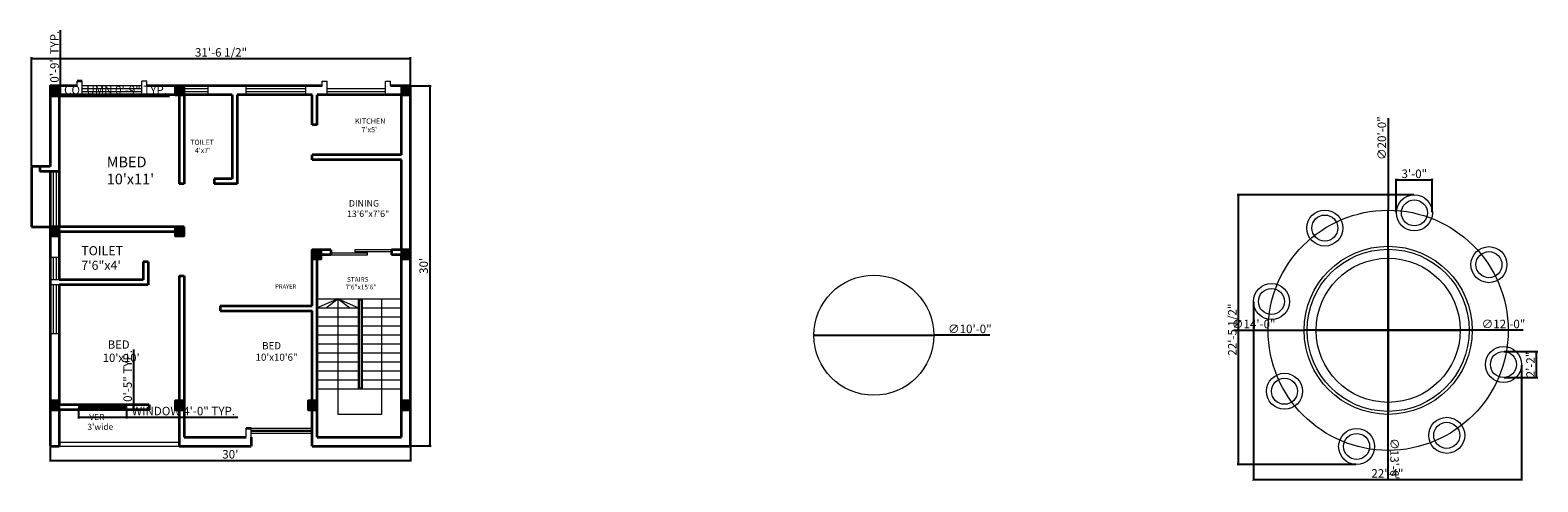
# Model space of a CAD drawing. Units: inches. Extents: x 3799 to 20199, y 1682 to 8087.
# Tile 1 of 30: x 3799 to 5306, y 1682 to 2133. Entities that reach past the tile are written whole.
import ezdxf

# ---------------------------------------------------------------- set-up
doc = ezdxf.new("R2010")
doc.units = ezdxf.units.IN
for name, color, linetype, lineweight in [('A-ANNO-DIMS', 2, 'Continuous', 18), ('A-AREA-IDEN', 7, 'Continuous', 18), ('A-COLS', 251, 'Continuous', 35), ('A-DETL', 7, 'Continuous', 18), ('A-DOOR', 3, 'Continuous', 18), ('A-FLOR-RAIL', 217, 'Continuous', 18), ('A-FLOR-STRS', 41, 'Continuous', 18), ('A-GLAZ', 152, 'Continuous', 18), ('A-WALL', 7, 'Continuous', 35)]:
    doc.layers.add(name, color=color, linetype=linetype, lineweight=lineweight)
doc.styles.get("Standard").update_dxf_attribs({"font": 'arial.ttf'})
doc.dimstyles.new('ISO-25', dxfattribs={"dimtxt": 8.5, "dimasz": 2.5, "dimexe": 1.25, "dimexo": 0.625, "dimtad": 1, "dimdec": 0, "dimlunit": 3, "dimtxsty": 'Standard', "dimblk": 'ARCHTICK', "dimcen": 2.5, "dimadec": 0, "dimazin": 0, "dimtfac": 1, "dimtdec": 0, "dimtmove": 0, "dimatfit": 3, "dimfxl": 1, "dimarcsym": 0})

# ---------------------------------------------------------------- blocks, each defined once
blk = doc.blocks.new('_ArchTick')
at = {"color": 0, "linetype": 'ByBlock', "const_width": 0.15}
blk.add_lwpolyline([(-0.5, -0.5), (0.5, 0.5)], dxfattribs=at)
blk = doc.blocks.new('*D2')
at = {"layer": 'A-ANNO-DIMS', "color": 0, "lineweight": -2, "transparency": 16777216}
for p, q in [((3818.8, 1716.8), (3818.8, 1701.9)), ((3818.8, 1703.1), (4178.8, 1703.1)), ((4178.8, 1716.8), (4178.8, 1701.9))]:
    blk.add_line(p, q, dxfattribs=at)
at = {"layer": 'Defpoints', "color": 0, "transparency": 16777216}
for p in [(3818.8, 1717.5), (4178.8, 1717.5), (4178.8, 1703.1)]:
    blk.add_point(p, dxfattribs=at)
at = {"layer": 'A-ANNO-DIMS', "color": 0, "lineweight": -2, "transparency": 16777216, "xscale": 2.5, "yscale": 2.5, "zscale": 2.5, "rotation": 180}
blk.add_blockref('_ArchTick', (3818.8, 1703.1), dxfattribs=at)
at = {"layer": 'A-ANNO-DIMS', "color": 0, "lineweight": -2, "transparency": 16777216, "xscale": 2.5, "yscale": 2.5, "zscale": 2.5}
blk.add_blockref('_ArchTick', (4178.8, 1703.1), dxfattribs=at)
at = {"layer": 'A-ANNO-DIMS', "color": 0, "transparency": 16777216, "insert": (3998.8, 1708.1), "char_height": 8.5, "attachment_point": 5}
blk.add_mtext("30'", dxfattribs=at)
blk = doc.blocks.new('*D3')
at = {"layer": 'A-ANNO-DIMS', "color": 0, "lineweight": -2, "transparency": 16777216}
for p, q in [((4179.4, 2077.5), (4199.4, 2077.5)), ((4198.2, 2077.5), (4198.2, 1717.5)), ((4179.4, 1717.5), (4199.4, 1717.5))]:
    blk.add_line(p, q, dxfattribs=at)
at = {"layer": 'Defpoints', "color": 0, "transparency": 16777216}
for p in [(4178.8, 2077.5), (4178.8, 1717.5), (4198.2, 1717.5)]:
    blk.add_point(p, dxfattribs=at)
at = {"layer": 'A-ANNO-DIMS', "color": 0, "lineweight": -2, "transparency": 16777216, "xscale": 2.5, "yscale": 2.5, "zscale": 2.5}
for p, rotation in [((4198.2, 2077.5), 90), ((4198.2, 1717.5), 270)]:
    blk.add_blockref('_ArchTick', p, dxfattribs=dict(at, rotation=rotation))
at = {"layer": 'A-ANNO-DIMS', "color": 0, "transparency": 16777216, "insert": (4193.2, 1897.5), "char_height": 8.5, "attachment_point": 5, "rotation": 90}
blk.add_mtext("30'", dxfattribs=at)
blk = doc.blocks.new('*U4')
for radius in [18, 13]:
    blk.add_circle((65.6, 19.3), radius)
blk = doc.blocks.new('*U5')
at = {"layer": 'A-DETL', "color": 0, "linetype": 'ByBlock', "lineweight": -2, "transparency": 16777216}
for p, rotation in [((5241.8, 1917), 134.3437921616318), ((5158.7, 1953.1), 178.6875843232637), ((5276, 1833.1), 90), ((5074.1, 1920.8), 223.0313764848954), ((5233.7, 1741.7), 40.40654513142267), ((5036.1, 1838.6), 267.3751686465272), ((5066.4, 1753.2), 311.718960808159), ((5147.7, 1713.4), 356.062752969791)]:
    blk.add_blockref('*U4', p, dxfattribs=dict(at, rotation=rotation))
blk = doc.blocks.new('WIN-48IN-5IN-FRAME')
for p, q in [((0, 5), (0, 0)), ((48, 3), (0, 3)), ((48, 2), (0, 2)), ((48, 5), (48, 0))]:
    blk.add_line(p, q)
blk = doc.blocks.new('COL-9X9IN')
h = blk.add_hatch(color=256)
h.dxf.hatch_style = 1
h.paths.add_polyline_path([(9, 9), (0, 9), (0, 0), (9, 0)])
blk.add_lwpolyline([(9, 9), (0, 9), (0, 0), (9, 0)], close=True)
blk = doc.blocks.new('*D270')
at = {"layer": 'A-ANNO-DIMS', "color": 0, "lineweight": -2, "transparency": 16777216}
for p, q in [((3818.8, 2067.8), (3818.8, 2065.9)), ((3818.8, 2067.1), (3827.8, 2067.1)), ((3827.8, 2067.8), (3827.8, 2065.9)), ((3827.8, 2067.1), (3938, 2067.1))]:
    blk.add_line(p, q, dxfattribs=at)
at = {"layer": 'Defpoints', "color": 0, "transparency": 16777216}
for p in [(3818.8, 2068.5), (3827.8, 2068.5), (3827.8, 2067.1)]:
    blk.add_point(p, dxfattribs=at)
at = {"layer": 'A-ANNO-DIMS', "color": 0, "lineweight": -2, "transparency": 16777216, "xscale": 2.5, "yscale": 2.5, "zscale": 2.5, "rotation": 180}
blk.add_blockref('_ArchTick', (3818.8, 2067.1), dxfattribs=at)
at = {"layer": 'A-ANNO-DIMS', "color": 0, "lineweight": -2, "transparency": 16777216, "xscale": 2.5, "yscale": 2.5, "zscale": 2.5}
blk.add_blockref('_ArchTick', (3827.8, 2067.1), dxfattribs=at)
at = {"layer": 'A-ANNO-DIMS', "color": 0, "transparency": 16777216, "insert": (3884.1, 2072.1), "char_height": 8.5, "attachment_point": 5}
blk.add_mtext('COLUMN 0\'-9" TYP.', dxfattribs=at)
blk = doc.blocks.new('*D271')
at = {"layer": 'A-ANNO-DIMS', "color": 0, "lineweight": -2, "transparency": 16777216}
for p, q in [((3829.1, 2077.5), (3829.1, 2133)), ((3828.4, 2077.5), (3830.4, 2077.5)), ((3828.4, 2068.5), (3830.4, 2068.5)), ((3829.1, 2068.5), (3829.1, 2077.5))]:
    blk.add_line(p, q, dxfattribs=at)
at = {"layer": 'Defpoints', "color": 0, "transparency": 16777216}
for p in [(3827.8, 2077.5), (3827.8, 2068.5), (3829.1, 2077.5)]:
    blk.add_point(p, dxfattribs=at)
at = {"layer": 'A-ANNO-DIMS', "color": 0, "lineweight": -2, "transparency": 16777216, "xscale": 2.5, "yscale": 2.5, "zscale": 2.5}
for p, rotation in [((3829.1, 2077.5), 90), ((3829.1, 2068.5), 270)]:
    blk.add_blockref('_ArchTick', p, dxfattribs=dict(at, rotation=rotation))
at = {"layer": 'A-ANNO-DIMS', "color": 0, "transparency": 16777216, "insert": (3824.2, 2106.5), "char_height": 8.5, "attachment_point": 5, "rotation": 90}
blk.add_mtext('0\'-9" TYP.', dxfattribs=at)
blk = doc.blocks.new('*D324')
at = {"layer": 'A-ANNO-DIMS', "color": 0, "lineweight": -2, "transparency": 16777216}
for p, q in [((3847.1, 1752.8), (3847.1, 1745)), ((3895.1, 1752.8), (3895.1, 1745)), ((3847.1, 1746.3), (3895.1, 1746.3)), ((3895.1, 1746.3), (4006.4, 1746.3))]:
    blk.add_line(p, q, dxfattribs=at)
at = {"layer": 'Defpoints', "color": 0, "transparency": 16777216}
for p in [(3847.1, 1753.5), (3895.1, 1753.5), (3895.1, 1746.3)]:
    blk.add_point(p, dxfattribs=at)
at = {"layer": 'A-ANNO-DIMS', "color": 0, "lineweight": -2, "transparency": 16777216, "xscale": 2.5, "yscale": 2.5, "zscale": 2.5, "rotation": 180}
blk.add_blockref('_ArchTick', (3847.1, 1746.3), dxfattribs=at)
at = {"layer": 'A-ANNO-DIMS', "color": 0, "lineweight": -2, "transparency": 16777216, "xscale": 2.5, "yscale": 2.5, "zscale": 2.5}
blk.add_blockref('_ArchTick', (3895.1, 1746.3), dxfattribs=at)
at = {"layer": 'A-ANNO-DIMS', "color": 0, "transparency": 16777216, "insert": (3952, 1751.3), "char_height": 8.5, "attachment_point": 5}
blk.add_mtext('WINDOW 4\'-0" TYP.', dxfattribs=at)
blk = doc.blocks.new('*D325')
at = {"layer": 'A-ANNO-DIMS', "color": 0, "lineweight": -2, "transparency": 16777216}
for p, q in [((3902.3, 1758.5), (3902.3, 1814)), ((3895.7, 1758.5), (3903.6, 1758.5)), ((3895.7, 1753.5), (3903.6, 1753.5)), ((3902.3, 1753.5), (3902.3, 1758.5))]:
    blk.add_line(p, q, dxfattribs=at)
at = {"layer": 'Defpoints', "color": 0, "transparency": 16777216}
for p in [(3895.1, 1758.5), (3895.1, 1753.5), (3902.3, 1758.5)]:
    blk.add_point(p, dxfattribs=at)
at = {"layer": 'A-ANNO-DIMS', "color": 0, "lineweight": -2, "transparency": 16777216, "xscale": 2.5, "yscale": 2.5, "zscale": 2.5}
for p, rotation in [((3902.3, 1758.5), 90), ((3902.3, 1753.5), 270)]:
    blk.add_blockref('_ArchTick', p, dxfattribs=dict(at, rotation=rotation))
at = {"layer": 'A-ANNO-DIMS', "color": 0, "transparency": 16777216, "insert": (3897.3, 1787.5), "char_height": 8.5, "attachment_point": 5, "rotation": 90}
blk.add_mtext('0\'-5" TYP.', dxfattribs=at)
blk = doc.blocks.new('*D360')
at = {"layer": 'A-ANNO-DIMS', "color": 0, "lineweight": -2, "transparency": 16777216}
for p, q in [((5164.1, 1951), (5164.1, 1984.6)), ((5164.1, 1983.4), (5200.1, 1983.4)), ((5200.1, 1951), (5200.1, 1984.6))]:
    blk.add_line(p, q, dxfattribs=at)
at = {"layer": 'Defpoints', "color": 0, "transparency": 16777216}
for p in [(5200.1, 1983.4), (5164.1, 1950.4), (5200.1, 1950.4)]:
    blk.add_point(p, dxfattribs=at)
at = {"layer": 'A-ANNO-DIMS', "color": 0, "lineweight": -2, "transparency": 16777216, "xscale": 2.5, "yscale": 2.5, "zscale": 2.5, "rotation": 180}
blk.add_blockref('_ArchTick', (5164.1, 1983.4), dxfattribs=at)
at = {"layer": 'A-ANNO-DIMS', "color": 0, "lineweight": -2, "transparency": 16777216, "xscale": 2.5, "yscale": 2.5, "zscale": 2.5}
blk.add_blockref('_ArchTick', (5200.1, 1983.4), dxfattribs=at)
at = {"layer": 'A-ANNO-DIMS', "color": 0, "transparency": 16777216, "insert": (5182.1, 1988.4), "char_height": 8.5, "attachment_point": 5}
blk.add_mtext('3\'-0"', dxfattribs=at)
blk = doc.blocks.new('*D361')
at = {"layer": 'A-ANNO-DIMS', "color": 0, "lineweight": -2, "transparency": 16777216}
for p, q in [((5271.8, 1811.9), (5305.4, 1811.9)), ((5304.2, 1785.9), (5304.2, 1811.9)), ((5271.8, 1785.9), (5305.4, 1785.9))]:
    blk.add_line(p, q, dxfattribs=at)
at = {"layer": 'Defpoints', "color": 0, "transparency": 16777216}
for p in [(5271.2, 1811.9), (5304.2, 1811.9), (5271.2, 1785.9)]:
    blk.add_point(p, dxfattribs=at)
at = {"layer": 'A-ANNO-DIMS', "color": 0, "lineweight": -2, "transparency": 16777216, "xscale": 2.5, "yscale": 2.5, "zscale": 2.5}
for p, rotation in [((5304.2, 1811.9), 90), ((5304.2, 1785.9), 270)]:
    blk.add_blockref('_ArchTick', p, dxfattribs=dict(at, rotation=rotation))
at = {"layer": 'A-ANNO-DIMS', "color": 0, "transparency": 16777216, "insert": (5299.3, 1798.9), "char_height": 8.5, "attachment_point": 5, "rotation": 90}
blk.add_mtext('2\'-2"', dxfattribs=at)
blk = doc.blocks.new('*D362')
at = {"layer": 'A-ANNO-DIMS', "color": 0, "lineweight": -2, "transparency": 16777216}
for p, q in [((5021.3, 1861.4), (5021.3, 1682.9)), ((5289.2, 1798.3), (5289.2, 1682.9)), ((5021.3, 1684.1), (5289.2, 1684.1))]:
    blk.add_line(p, q, dxfattribs=at)
at = {"layer": 'Defpoints', "color": 0, "transparency": 16777216}
for p in [(5021.3, 1862), (5289.2, 1798.9), (5289.2, 1684.1)]:
    blk.add_point(p, dxfattribs=at)
at = {"layer": 'A-ANNO-DIMS', "color": 0, "lineweight": -2, "transparency": 16777216, "xscale": 2.5, "yscale": 2.5, "zscale": 2.5, "rotation": 180}
blk.add_blockref('_ArchTick', (5021.3, 1684.1), dxfattribs=at)
at = {"layer": 'A-ANNO-DIMS', "color": 0, "lineweight": -2, "transparency": 16777216, "xscale": 2.5, "yscale": 2.5, "zscale": 2.5}
blk.add_blockref('_ArchTick', (5289.2, 1684.1), dxfattribs=at)
at = {"layer": 'A-ANNO-DIMS', "color": 0, "transparency": 16777216, "insert": (5155.2, 1689), "char_height": 8.5, "attachment_point": 5}
blk.add_mtext('22\'-4"', dxfattribs=at)
blk = doc.blocks.new('*D363')
at = {"layer": 'A-ANNO-DIMS', "color": 0, "lineweight": -2, "transparency": 16777216}
for p, q in [((5181.5, 1968.4), (5005, 1968.4)), ((5006.3, 1699.1), (5006.3, 1968.4)), ((5123.8, 1699.1), (5005, 1699.1))]:
    blk.add_line(p, q, dxfattribs=at)
at = {"layer": 'Defpoints', "color": 0, "transparency": 16777216}
for p in [(5006.3, 1968.4), (5182.1, 1968.4), (5124.4, 1699.1)]:
    blk.add_point(p, dxfattribs=at)
at = {"layer": 'A-ANNO-DIMS', "color": 0, "lineweight": -2, "transparency": 16777216, "xscale": 2.5, "yscale": 2.5, "zscale": 2.5}
for p, rotation in [((5006.3, 1968.4), 90), ((5006.3, 1699.1), 270)]:
    blk.add_blockref('_ArchTick', p, dxfattribs=dict(at, rotation=rotation))
at = {"layer": 'A-ANNO-DIMS', "color": 0, "transparency": 16777216, "insert": (5001.3, 1833.8), "char_height": 8.5, "attachment_point": 5, "rotation": 90}
blk.add_mtext('22\'-5 1/2"', dxfattribs=at)
blk = doc.blocks.new('*D366')
at = {"layer": 'A-ANNO-DIMS', "color": 0, "lineweight": -2, "transparency": 16777216}
for p, q in [((3800.2, 1997.5), (3800.2, 2105.9)), ((3800.2, 2104.7), (4178.8, 2104.7)), ((4178.8, 2078.1), (4178.8, 2105.9))]:
    blk.add_line(p, q, dxfattribs=at)
at = {"layer": 'Defpoints', "color": 0, "transparency": 16777216}
for p in [(4178.8, 2104.7), (4178.8, 2077.5), (3800.2, 1996.9)]:
    blk.add_point(p, dxfattribs=at)
at = {"layer": 'A-ANNO-DIMS', "color": 0, "lineweight": -2, "transparency": 16777216, "xscale": 2.5, "yscale": 2.5, "zscale": 2.5, "rotation": 180}
blk.add_blockref('_ArchTick', (3800.2, 2104.7), dxfattribs=at)
at = {"layer": 'A-ANNO-DIMS', "color": 0, "lineweight": -2, "transparency": 16777216, "xscale": 2.5, "yscale": 2.5, "zscale": 2.5}
blk.add_blockref('_ArchTick', (4178.8, 2104.7), dxfattribs=at)
at = {"layer": 'A-ANNO-DIMS', "color": 0, "transparency": 16777216, "insert": (3989.5, 2109.7), "char_height": 8.5, "attachment_point": 5}
blk.add_mtext('31\'-6 1/2"', dxfattribs=at)
blk = doc.blocks.new('*D379')
at = {"layer": 'A-ANNO-DIMS', "color": 0, "lineweight": -2, "transparency": 16777216}
for p in [(4581.9, 1828.2), (4757.8, 1828.2)]:
    blk.add_line(p, (4701.9, 1828.2), dxfattribs=at)
at = {"layer": 'Defpoints', "color": 0, "transparency": 16777216}
for p in [(4581.9, 1828.2), (4701.9, 1828.2)]:
    blk.add_point(p, dxfattribs=at)
at = {"layer": 'A-ANNO-DIMS', "color": 0, "lineweight": -2, "transparency": 16777216, "xscale": 2.5, "yscale": 2.5, "zscale": 2.5}
for p, rotation in [((4581.9, 1828.2), 359.9997507633592), ((4701.9, 1828.2), 179.9997507633592)]:
    blk.add_blockref('_ArchTick', p, dxfattribs=dict(at, rotation=rotation))
at = {"layer": 'A-ANNO-DIMS', "color": 0, "transparency": 16777216, "insert": (4737.9, 1833.4), "char_height": 8.5, "attachment_point": 5, "rotation": 359.9998}
blk.add_mtext('∅10\'-0"', dxfattribs=at)
blk = doc.blocks.new('*D380')
at = {"layer": 'A-ANNO-DIMS', "color": 0, "lineweight": -2, "transparency": 16777216}
for p in [(5156, 2045), (5156, 1713.1)]:
    blk.add_line(p, (5156, 1953.1), dxfattribs=at)
at = {"layer": 'Defpoints', "color": 0, "transparency": 16777216}
for p in [(5156, 1953.1), (5156, 1713.1)]:
    blk.add_point(p, dxfattribs=at)
at = {"layer": 'A-ANNO-DIMS', "color": 0, "lineweight": -2, "transparency": 16777216, "xscale": 2.5, "yscale": 2.5, "zscale": 2.5}
for p, rotation in [((5156, 1953.1), 270), ((5156, 1713.1), 90)]:
    blk.add_blockref('_ArchTick', p, dxfattribs=dict(at, rotation=rotation))
at = {"layer": 'A-ANNO-DIMS', "color": 0, "transparency": 16777216, "insert": (5150.7, 2025.1), "char_height": 8.5, "attachment_point": 5, "rotation": 90}
blk.add_mtext('∅20\'-0"', dxfattribs=at)
blk = doc.blocks.new('*D381')
at = {"layer": 'A-ANNO-DIMS', "color": 0, "lineweight": -2, "transparency": 16777216}
for p in [(5001.7, 1833.1), (5240, 1833.1)]:
    blk.add_line(p, (5072, 1833.1), dxfattribs=at)
at = {"layer": 'Defpoints', "color": 0, "transparency": 16777216}
for p in [(5072, 1833.1), (5240, 1833.1)]:
    blk.add_point(p, dxfattribs=at)
at = {"layer": 'A-ANNO-DIMS', "color": 0, "lineweight": -2, "transparency": 16777216, "xscale": 2.5, "yscale": 2.5, "zscale": 2.5}
blk.add_blockref('_ArchTick', (5072, 1833.1), dxfattribs=at)
at = {"layer": 'A-ANNO-DIMS', "color": 0, "lineweight": -2, "transparency": 16777216, "xscale": 2.5, "yscale": 2.5, "zscale": 2.5, "rotation": 180}
blk.add_blockref('_ArchTick', (5240, 1833.1), dxfattribs=at)
at = {"layer": 'A-ANNO-DIMS', "color": 0, "transparency": 16777216, "insert": (5021.6, 1838.3), "char_height": 8.5, "attachment_point": 5}
blk.add_mtext('∅14\'-0"', dxfattribs=at)
blk = doc.blocks.new('*D382')
at = {"layer": 'A-ANNO-DIMS', "color": 0, "lineweight": -2, "transparency": 16777216}
for p in [(5156, 1914.1), (5156, 1683.7)]:
    blk.add_line(p, (5156, 1752.1), dxfattribs=at)
at = {"layer": 'Defpoints', "color": 0, "transparency": 16777216}
for p in [(5156, 1914.1), (5156, 1752.1)]:
    blk.add_point(p, dxfattribs=at)
at = {"layer": 'A-ANNO-DIMS', "color": 0, "lineweight": -2, "transparency": 16777216, "xscale": 2.5, "yscale": 2.5, "zscale": 2.5}
for p, rotation in [((5156, 1914.1), 270.0000643693325), ((5156, 1752.1), 90.00006436933245)]:
    blk.add_blockref('_ArchTick', p, dxfattribs=dict(at, rotation=rotation))
at = {"layer": 'A-ANNO-DIMS', "color": 0, "transparency": 16777216, "insert": (5161.2, 1703.5), "char_height": 8.5, "attachment_point": 5, "rotation": 270.0001}
blk.add_mtext('∅13\'-6"', dxfattribs=at)
blk = doc.blocks.new('*D383')
at = {"layer": 'A-ANNO-DIMS', "color": 0, "lineweight": -2, "transparency": 16777216}
for p in [(5084, 1833.1), (5291, 1833.1)]:
    blk.add_line(p, (5228, 1833.1), dxfattribs=at)
at = {"layer": 'Defpoints', "color": 0, "transparency": 16777216}
for p in [(5084, 1833.1), (5228, 1833.1)]:
    blk.add_point(p, dxfattribs=at)
at = {"layer": 'A-ANNO-DIMS', "color": 0, "lineweight": -2, "transparency": 16777216, "xscale": 2.5, "yscale": 2.5, "zscale": 2.5}
for p, rotation in [((5084, 1833.1), 359.9999514577424), ((5228, 1833.1), 179.9999514577424)]:
    blk.add_blockref('_ArchTick', p, dxfattribs=dict(at, rotation=rotation))
at = {"layer": 'A-ANNO-DIMS', "color": 0, "transparency": 16777216, "insert": (5271.2, 1838.3), "char_height": 8.5, "attachment_point": 5, "rotation": 360}
blk.add_mtext('∅12\'-0"', dxfattribs=at)

msp = doc.modelspace()

# ---------------------------------------------------------------- linework, layer by layer
at = {"layer": 'A-DETL'}
for centre, radius in [((5155.95, 1833.1), 120), ((5155.95, 1833.1), 84), ((5155.95, 1833.1), 81), ((5155.95, 1833.1), 72), ((4641.93, 1828.16), 60)]:
    msp.add_circle(centre, radius, dxfattribs=at)
at = {"layer": 'A-DOOR'}
for p, q in [((4099.28, 1910.47), (4135.83, 1910.47)), ((4099.28, 1908.47), (4135.83, 1908.47)), ((4159.93, 1913.47), (4123.17, 1913.47)), ((4123.17, 1913.47), (4123.17, 1911.47)), ((4159.93, 1911.47), (4123.17, 1911.47)), ((4135.83, 1908.47), (4135.83, 1910.47))]:
    msp.add_line(p, q, dxfattribs=at)
at = {"layer": 'A-FLOR-RAIL'}
for p, q in [((3827.77, 1721.47), (3947.77, 1721.47)), ((3827.77, 1717.47), (3947.77, 1717.47))]:
    msp.add_line(p, q, dxfattribs=at)
at = {"layer": 'A-FLOR-STRS'}
for p, q in [((4085.77, 1864.58), (4169.77, 1864.58)), ((4106.74, 1864.58), (4085.77, 1855.58)), ((4085.77, 1855.58), (4126.77, 1855.58)), ((4106.74, 1864.58), (4094.8, 1855.58)), ((4106.74, 1748.85), (4106.74, 1864.58)), ((4106.74, 1864.58), (4126.77, 1855.58)), ((4106.74, 1864.58), (4118.34, 1855.58)), ((4126.77, 1774.58), (4126.77, 1864.58)), ((4127.77, 1775.58), (4127.77, 1863.58)), ((4127.77, 1863.58), (4129.77, 1863.58)), ((4129.77, 1775.58), (4129.77, 1863.58)), ((4130.77, 1774.58), (4130.77, 1864.58)), ((4130.77, 1855.58), (4169.77, 1855.58)), ((4150.03, 1864.58), (4150.03, 1748.85)), ((4085.77, 1846.58), (4126.77, 1846.58)), ((4130.77, 1846.58), (4169.77, 1846.58)), ((4085.77, 1837.58), (4126.77, 1837.58)), ((4085.77, 1828.58), (4126.77, 1828.58)), ((4130.77, 1837.58), (4169.77, 1837.58)), ((4130.77, 1828.58), (4169.77, 1828.58)), ((4085.77, 1819.58), (4126.77, 1819.58)), ((4085.77, 1810.58), (4126.77, 1810.58)), ((4130.77, 1819.58), (4169.77, 1819.58)), ((4130.77, 1810.58), (4169.77, 1810.58)), ((4085.77, 1801.58), (4126.77, 1801.58)), ((4130.77, 1801.58), (4169.77, 1801.58)), ((4085.77, 1792.58), (4126.77, 1792.58)), ((4085.77, 1783.58), (4126.77, 1783.58)), ((4130.77, 1792.58), (4169.77, 1792.58)), ((4130.77, 1783.58), (4169.77, 1783.58)), ((4085.77, 1774.58), (4169.77, 1774.58)), ((4127.77, 1775.58), (4129.77, 1775.58)), ((4150.03, 1748.85), (4106.74, 1748.85))]:
    msp.add_line(p, q, dxfattribs=at)
at = {"layer": 'A-GLAZ'}
for p, q in [((3845.89, 2077.47), (3845.89, 2082.18)), ((3850.89, 2068.47), (3850.89, 2082.18)), ((3910.28, 2068.47), (3910.28, 2082.18)), ((3915.28, 2082.18), (3910.28, 2082.18)), ((3915.28, 2077.47), (3915.28, 2082.18)), ((4090.62, 2077.47), (4090.62, 2082.18)), ((4090.62, 2082.18), (4095.62, 2082.18)), ((4095.62, 2068.47), (4095.62, 2082.18)), ((4154.03, 2068.47), (4154.03, 2082.18)), ((4154.03, 2082.18), (4159.03, 2082.18)), ((4159.03, 2077.47), (4159.03, 2082.18)), ((3910.28, 2077.47), (3850.89, 2077.47)), ((3910.28, 2074.47), (3850.89, 2074.47)), ((3910.28, 2071.47), (3850.89, 2071.47)), ((3976.33, 2074.47), (3952.75, 2074.47)), ((3976.33, 2071.47), (3952.77, 2071.47)), ((3976.33, 2077.47), (3976.33, 2068.47)), ((4014.74, 2068.47), (4014.74, 2077.47)), ((4074.26, 2074.47), (4014.74, 2074.47)), ((4074.26, 2071.47), (4014.74, 2071.47)), ((4074.26, 2068.47), (4074.26, 2077.47)), ((4154.03, 2074.47), (4095.62, 2074.47)), ((4154.03, 2071.47), (4095.62, 2071.47)), ((3821.77, 1991.87), (3821.77, 1936.47)), ((3824.77, 1991.87), (3824.77, 1936.47)), ((3827.77, 1905.89), (3818.77, 1905.89)), ((3821.77, 1905.89), (3821.77, 1883.47)), ((3824.77, 1905.89), (3824.77, 1883.47)), ((3827.77, 1883.47), (3818.77, 1883.47)), ((3827.77, 1878.47), (3818.77, 1878.47)), ((3821.77, 1878.47), (3821.77, 1829.54)), ((3824.77, 1878.47), (3824.77, 1829.54)), ((3827.77, 1829.54), (3818.77, 1829.54)), ((4014.77, 1726.47), (4014.77, 1735.44)), ((4019.77, 1726.47), (4019.77, 1735.44)), ((4019.77, 1735.44), (4080.77, 1735.44)), ((4019.77, 1733.44), (4080.77, 1733.44)), ((4019.77, 1732.44), (4080.77, 1732.44)), ((4019.77, 1730.44), (4080.77, 1730.44))]:
    msp.add_line(p, q, dxfattribs=at)
at = {"layer": 'A-WALL'}
for p, q in [((3850.89, 2082.18), (3845.89, 2082.18)), ((3818.77, 2077.47), (3818.77, 1996.87)), ((3845.89, 2077.47), (3818.77, 2077.47)), ((3821.77, 2077.47), (3821.77, 2068.47)), ((3827.77, 2068.47), (3827.77, 1936.47)), ((3947.77, 2068.47), (3827.77, 2068.47)), ((4090.62, 2077.47), (3915.28, 2077.47)), ((3947.77, 2068.47), (3947.77, 1979.47)), ((3952.77, 2068.47), (3952.77, 1984.47)), ((4000.77, 2068.47), (3952.77, 2068.47)), ((4000.77, 2068.47), (4000.77, 1984.47)), ((4005.77, 2068.47), (4005.77, 1979.47)), ((4080.77, 2068.47), (4005.77, 2068.47)), ((4080.77, 2038.47), (4080.77, 2068.47)), ((4169.77, 2068.47), (4085.77, 2068.47)), ((4085.77, 2038.47), (4085.77, 2068.47)), ((4178.77, 2077.47), (4159.03, 2077.47)), ((4178.77, 2074.47), (4169.77, 2074.47)), ((4169.77, 2008.47), (4169.77, 2068.47)), ((4178.77, 1717.47), (4178.77, 2077.47)), ((4085.77, 2038.47), (4080.77, 2038.47)), ((4080.77, 2003.47), (4080.77, 2008.47)), ((4085.77, 2008.47), (4080.77, 2008.47)), ((4169.77, 2008.47), (4085.77, 2008.47)), ((3808.35, 1996.87), (3800.15, 1996.87)), ((3800.15, 1996.87), (3800.15, 1936.47)), ((3818.77, 1996.87), (3808.35, 1996.87)), ((3808.35, 1996.87), (3808.35, 1991.87)), ((3827.77, 1991.87), (3808.35, 1991.87)), ((3818.77, 1991.87), (3818.77, 1717.47)), ((4169.77, 2003.47), (4080.77, 2003.47)), ((4169.77, 1913.47), (4169.77, 2003.47)), ((3952.77, 1979.47), (3947.77, 1979.47)), ((3952.77, 1984.47), (3952.77, 1979.47)), ((4000.77, 1984.47), (3982.77, 1984.47)), ((3982.77, 1984.47), (3982.77, 1979.47)), ((4005.77, 1979.47), (3982.77, 1979.47)), ((3800.15, 1936.47), (3818.77, 1936.47)), ((3952.77, 1936.47), (3827.77, 1936.47)), ((3952.77, 1931.47), (3827.77, 1931.47)), ((3827.77, 1931.47), (3827.77, 1883.47)), ((3952.77, 1931.47), (3952.77, 1936.47)), ((3911.77, 1901.47), (3911.77, 1883.47)), ((3916.77, 1901.47), (3911.77, 1901.47)), ((3916.77, 1901.47), (3916.77, 1878.47)), ((4080.77, 1857.47), (4080.77, 1913.47)), ((4099.28, 1913.47), (4080.77, 1913.47)), ((4085.77, 1726.47), (4085.77, 1908.47)), ((4099.28, 1908.47), (4085.77, 1908.47)), ((4099.28, 1913.47), (4099.28, 1908.47)), ((4169.77, 1913.47), (4159.93, 1913.47)), ((4159.93, 1913.47), (4159.93, 1908.47)), ((4169.77, 1908.47), (4159.93, 1908.47)), ((4169.77, 1726.47), (4169.77, 1908.47)), ((3947.77, 1887.43), (3947.77, 1758.47)), ((3947.77, 1887.43), (3952.77, 1887.43)), ((3952.77, 1887.43), (3952.77, 1726.47)), ((3911.77, 1883.47), (3827.77, 1883.47)), ((3916.77, 1878.47), (3827.77, 1878.47)), ((3827.77, 1878.47), (3827.77, 1758.47)), ((3988.77, 1857.47), (4080.77, 1857.47)), ((3988.77, 1857.47), (3988.77, 1852.47)), ((3988.77, 1852.47), (4080.77, 1852.47)), ((4080.77, 1717.47), (4080.77, 1852.47)), ((3917.77, 1758.47), (3827.77, 1758.47)), ((3917.77, 1753.47), (3827.77, 1753.47)), ((3827.77, 1753.47), (3827.77, 1722.47)), ((3917.77, 1758.47), (3917.77, 1753.47)), ((3947.77, 1758.47), (3947.77, 1753.47)), ((3947.77, 1753.47), (3947.77, 1717.47)), ((4014.77, 1735.44), (4019.77, 1735.44)), ((3827.77, 1722.47), (3827.77, 1717.47)), ((3952.77, 1726.47), (4014.77, 1726.47)), ((4019.77, 1726.47), (4019.77, 1717.47)), ((4085.77, 1726.47), (4169.77, 1726.47)), ((3818.77, 1717.47), (3827.77, 1717.47)), ((3947.77, 1717.47), (4019.77, 1717.47)), ((4080.77, 1717.47), (4178.77, 1717.47))]:
    msp.add_line(p, q, dxfattribs=at)

# ---------------------------------------------------------------- block references
at = {"layer": 'A-COLS'}
for p in [(3818.77, 2068.47), (3943.75, 2068.47), (4169.77, 2068.47), (3818.77, 1927.47), (3943.78, 1927.47), (4080.77, 1904.37), (4169.77, 1904.47), (3818.77, 1753.47), (3943.77, 1753.47), (4076.77, 1753.47), (4169.77, 1753.47)]:
    msp.add_blockref('COL-9X9IN', p, dxfattribs=at)
at = {"layer": 'A-DETL'}
msp.add_blockref('*U5', (0, 0), dxfattribs=at)
at = {"layer": 'A-GLAZ'}
msp.add_blockref('WIN-48IN-5IN-FRAME', (3847.11, 1753.47), dxfattribs=at)

# ---------------------------------------------------------------- texts
at = {"layer": 'A-AREA-IDEN'}
for s, height, p in [('KITCHEN', 5.296, (4123.41, 2039.49)), ("    7'x5'", 5.296, (4123.41, 2030.98)), ('TOILET', 5.117, (3958.78, 2018.46)), ('MBED', 10.616, (3875.31, 1995.98)), ("   4'x7'", 5.117, (3958.78, 2010.24)), ("10'x11'", 10.616, (3875.32, 1978.92)), (' DINING', 6.485, (4115.36, 1956.71)), ('13\'6"x7\'6"', 6.485, (4115.37, 1946.29)), ('TOILET', 9.087, (3849.85, 1908.11)), ('7\'6"x4\'', 9.087, (3849.85, 1893.52)), (' STAIRS', 4.733, (4113.98, 1881.55)), ('PRAYER', 4.244, (4043.67, 1874.78)), ('7\'6"x15\'6"', 4.733, (4113.98, 1873.94)), ("10'x10'", 8.245, (3871.36, 1801.49)), ('  BED', 8.245, (3871.35, 1814.73)), ('10\'x10\'6"', 7.162, (4024.02, 1802.62)), ('   BED', 7.162, (4024.02, 1814.13)), (' VER', 6.14, (3855.95, 1743.45)), ("3'wide", 6.14, (3855.96, 1733.58))]:
    msp.add_text(s, height=height, rotation=0.03333, dxfattribs=at).set_placement(p)

# ---------------------------------------------------------------- dimensions: what is measured, and where the dimension line sits
at = {"layer": 'A-ANNO-DIMS'}
for base, p1, p2, picture, middle in [((3829.12, 2077.47), (3827.77, 2068.47), (3827.77, 2077.47), '*D271', (3824.16, 2106.51)), ((3902.31, 1758.47), (3895.11, 1753.47), (3895.11, 1758.47), '*D325', (3897.35, 1787.51))]:
    dim = msp.add_linear_dim(base=base, p1=p1, p2=p2, angle=90, text='<> TYP.', dimstyle='ISO-25', override={"dimdec": 1, "dimlfac": 1, "dimrnd": 0, "dimzin": 1, "dimdsep": 46, "dimlunit": 4, "dimfrac": 2}, dxfattribs=at)
    dim.commit()
    dim.dimension.update_dxf_attribs({"geometry": picture, "text_midpoint": middle})
for base, p1, p2, override, picture, middle in [((4178.77, 2104.68), (3800.15, 1996.87), (4178.77, 2077.47), {"dimdec": 1, "dimlfac": 1, "dimrnd": 0, "dimzin": 1, "dimdsep": 46, "dimlunit": 4, "dimfrac": 2}, '*D366', (3989.46, 2109.7)), ((5200.15, 1983.4), (5164.15, 1950.4), (5200.15, 1950.4), {"dimdec": 1, "dimlfac": 1, "dimrnd": 0, "dimzin": 1, "dimdsep": 46, "dimlunit": 4, "dimfrac": 2}, '*D360', (5182.15, 1988.36)), ((5289.17, 1684.13), (5021.29, 1861.98), (5289.17, 1798.92), {"dimdec": 1, "dimlfac": 1, "dimrnd": 0, "dimzin": 1, "dimdsep": 46, "dimlunit": 4, "dimfrac": 2}, '*D362', (5155.23, 1689.02)), ((4178.77, 1703.15), (3818.77, 1717.47), (4178.77, 1717.47), {"dimclrd": 0, "dimclre": 0, "dimclrt": 0}, '*D2', (3998.77, 1708.11))]:
    dim = msp.add_linear_dim(base=base, p1=p1, p2=p2, dimstyle='ISO-25', override=override, dxfattribs=at)
    dim.commit()
    dim.dimension.update_dxf_attribs({"geometry": picture, "text_midpoint": middle})
for base, p1, p2, text, picture, middle in [((3827.77, 2067.12), (3818.77, 2068.47), (3827.77, 2068.47), 'COLUMN <> TYP.', '*D270', (3884.13, 2072.15)), ((3895.11, 1746.27), (3847.11, 1753.47), (3895.11, 1753.47), 'WINDOW <> TYP.', '*D324', (3952.02, 1751.3))]:
    dim = msp.add_linear_dim(base=base, p1=p1, p2=p2, text=text, dimstyle='ISO-25', override={"dimdec": 1, "dimlfac": 1, "dimrnd": 0, "dimzin": 1, "dimdsep": 46, "dimlunit": 4, "dimfrac": 2}, dxfattribs=at)
    dim.commit()
    dim.dimension.update_dxf_attribs({"geometry": picture, "text_midpoint": middle})
for base, p1, p2, override, picture, middle in [((4198.17, 1717.47), (4178.77, 2077.47), (4178.77, 1717.47), {"dimclrd": 0, "dimclre": 0, "dimclrt": 0}, '*D3', (4193.2, 1897.47)), ((5006.29, 1968.4), (5124.41, 1699.13), (5182.15, 1968.4), {"dimdec": 1, "dimlfac": 1, "dimrnd": 0, "dimzin": 1, "dimdsep": 46, "dimlunit": 4, "dimfrac": 2}, '*D363', (5001.27, 1833.76)), ((5304.17, 1811.92), (5271.17, 1785.92), (5271.17, 1811.92), {"dimdec": 1, "dimlfac": 1, "dimrnd": 0, "dimzin": 1, "dimdsep": 46, "dimlunit": 4, "dimfrac": 2}, '*D361', (5299.28, 1798.92))]:
    dim = msp.add_linear_dim(base=base, p1=p1, p2=p2, angle=90, dimstyle='ISO-25', override=override, dxfattribs=at)
    dim.commit()
    dim.dimension.update_dxf_attribs({"geometry": picture, "text_midpoint": middle})
for p1, p2, picture, middle in [((5155.95, 1713.1), (5155.95, 1953.1), '*D380', (5155.95, 2025.1)), ((5155.95, 1914.1), (5155.95, 1752.1), '*D382', (5155.95, 1703.5)), ((4581.93, 1828.16), (4701.93, 1828.16), '*D379', (4737.93, 1828.16)), ((5239.95, 1833.1), (5071.95, 1833.1), '*D381', (5021.55, 1833.1)), ((5083.95, 1833.1), (5227.95, 1833.1), '*D383', (5271.15, 1833.1))]:
    dim = msp.add_diameter_dim_2p(p1=p1, p2=p2, dimstyle='ISO-25', override={"dimdec": 1, "dimlfac": 1, "dimrnd": 0, "dimzin": 1, "dimdsep": 46, "dimlunit": 4, "dimfrac": 2}, dxfattribs=at)
    dim.commit()
    dim.dimension.update_dxf_attribs({"geometry": picture, "text_midpoint": middle, "dimtype": 163})

doc.saveas('drawing.dxf')
